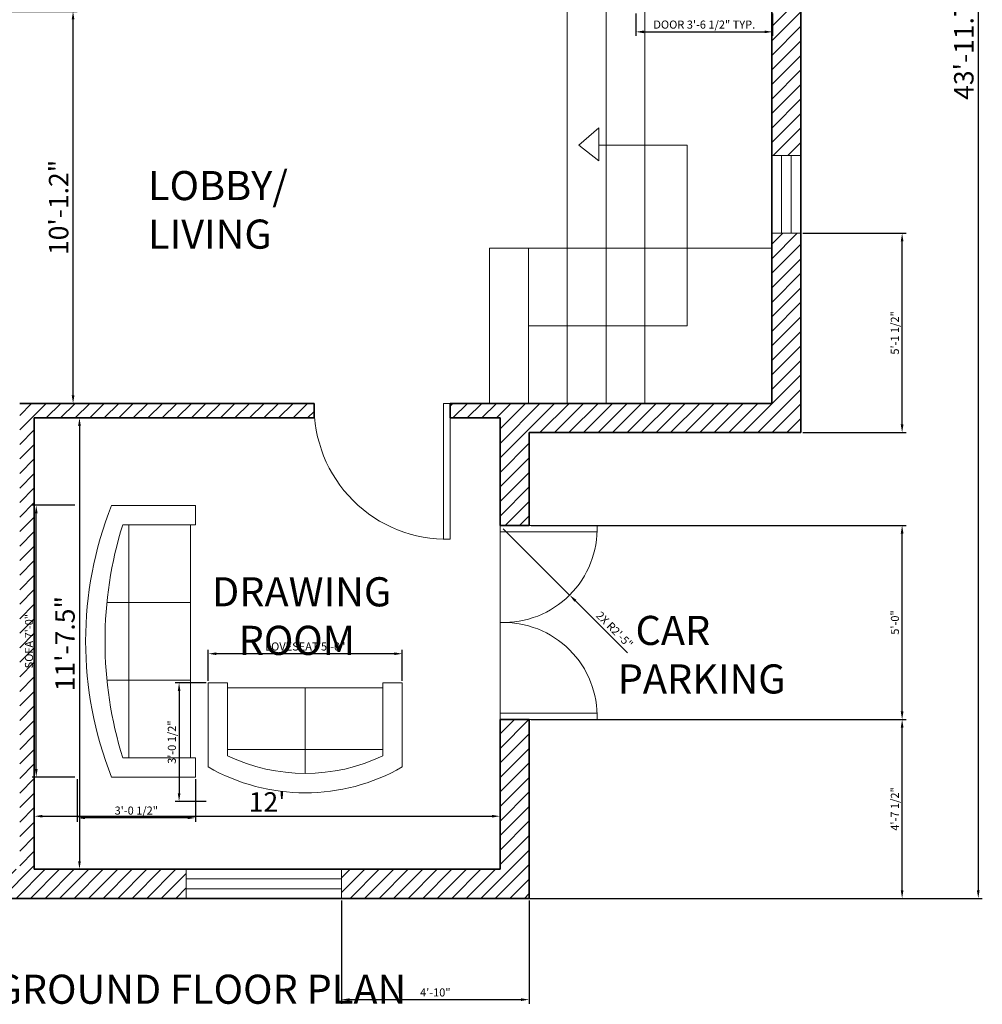
# Model space of a CAD drawing. Units: inches. Extents: x 4740 to 5323, y 7115 to 7713.
# Tile 2 of 6: x 5025 to 5323, y 7115 to 7420. Entities that reach past the tile are written whole.
import ezdxf

# ---------------------------------------------------------------- set-up
doc = ezdxf.new("R2010")
doc.units = ezdxf.units.IN
for name, color, linetype, lineweight in [('A-ANNO-DIMS', 2, 'Continuous', 18), ('A-ANNO-TEXT', 7, 'Continuous', 25), ('A-AREA-IDEN', 7, 'Continuous', 25), ('A-DOOR', 4, 'Continuous', 18), ('A-FLOR-STRS', 7, 'Continuous', 18), ('A-FURN', 8, 'Continuous', 18), ('A-GLAZ', 242, 'Continuous', 18), ('A-WALL', 7, 'Continuous', 35)]:
    doc.layers.add(name, color=color, linetype=linetype, lineweight=lineweight)
doc.layers.add('A-WALL-PATT', color=152, linetype='Continuous', lineweight=13, true_color=0x2776bb)
doc.styles.get("Standard").update_dxf_attribs({"font": 'arial.ttf'})
doc.dimstyles.new('ISO-25', dxfattribs={"dimtxt": 2.5, "dimasz": 2.5, "dimexe": 1.25, "dimexo": 0.625, "dimtad": 1, "dimlunit": 3, "dimtxsty": 'Standard', "dimcen": 2.5, "dimadec": 0, "dimazin": 0, "dimtfac": 1, "dimtmove": 0, "dimatfit": 3, "dimfxl": 1, "dimarcsym": 0})

# ---------------------------------------------------------------- blocks, each defined once
blk = doc.blocks.new('*D23')
at = {"layer": 'A-ANNO-DIMS', "color": 0, "lineweight": -2, "transparency": 16777216}
for p, q in [((5030.58, 7296.66), (5045.19, 7296.66)), ((5043.94, 7294.16), (5043.94, 7159.66)), ((5030.58, 7157.16), (5045.19, 7157.16))]:
    blk.add_line(p, q, dxfattribs=at)
at = {"layer": 'A-ANNO-DIMS', "color": 0, "transparency": 16777216}
for points in [[(5043.52, 7294.16), (5044.36, 7294.16), (5043.94, 7296.66)], [(5043.52, 7159.66), (5044.36, 7159.66), (5043.94, 7157.16)]]:
    blk.add_solid(points, dxfattribs=at)
at = {"layer": 'Defpoints', "color": 0, "transparency": 16777216}
for p in [(5029.96, 7296.66), (5029.96, 7157.16), (5043.94, 7157.16)]:
    blk.add_point(p, dxfattribs=at)
at = {"layer": 'A-ANNO-DIMS', "color": 0, "transparency": 16777216, "insert": (5040.25, 7226.91), "char_height": 6, "attachment_point": 5, "rotation": 90}
blk.add_mtext('11\'-7.5"', dxfattribs=at)
blk = doc.blocks.new('*D24')
at = {"layer": 'A-ANNO-DIMS', "color": 0, "lineweight": -2, "transparency": 16777216}
for p, q in [((5029.96, 7157.78), (5029.96, 7174.81)), ((5173.96, 7157.78), (5173.96, 7174.81)), ((5032.46, 7173.56), (5171.46, 7173.56))]:
    blk.add_line(p, q, dxfattribs=at)
at = {"layer": 'A-ANNO-DIMS', "color": 0, "transparency": 16777216}
for points in [[(5032.46, 7173.97), (5032.46, 7173.14), (5029.96, 7173.56)], [(5171.46, 7173.97), (5171.46, 7173.14), (5173.96, 7173.56)]]:
    blk.add_solid(points, dxfattribs=at)
at = {"layer": 'Defpoints', "color": 0, "transparency": 16777216}
for p in [(5173.96, 7173.56), (5029.96, 7157.16), (5173.96, 7157.16)]:
    blk.add_point(p, dxfattribs=at)
at = {"layer": 'A-ANNO-DIMS', "color": 0, "transparency": 16777216, "insert": (5101.96, 7177.19), "char_height": 6, "attachment_point": 5}
blk.add_mtext("12'", dxfattribs=at)
blk = doc.blocks.new('*D29')
at = {"layer": 'A-ANNO-DIMS', "color": 0, "lineweight": -2, "transparency": 16777216}
for p, q in [((5012.58, 7422.36), (5043.21, 7422.36)), ((5041.96, 7303.66), (5041.96, 7419.86)), ((5026.08, 7301.16), (5043.21, 7301.16))]:
    blk.add_line(p, q, dxfattribs=at)
at = {"layer": 'A-ANNO-DIMS', "color": 0, "transparency": 16777216}
for points in [[(5041.54, 7419.86), (5042.38, 7419.86), (5041.96, 7422.36)], [(5041.54, 7303.66), (5042.38, 7303.66), (5041.96, 7301.16)]]:
    blk.add_solid(points, dxfattribs=at)
at = {"layer": 'Defpoints', "color": 0, "transparency": 16777216}
for p in [(5011.96, 7422.36), (5041.96, 7422.36), (5025.46, 7301.16)]:
    blk.add_point(p, dxfattribs=at)
at = {"layer": 'A-ANNO-DIMS', "color": 0, "transparency": 16777216, "insert": (5038.27, 7361.76), "char_height": 6, "attachment_point": 5, "rotation": 90}
blk.add_mtext('10\'-1.2"', dxfattribs=at)
blk = doc.blocks.new('Sofa - Roundback 7 ft.')
for p, q in [((-12.00002, -32.4421), (-12.00003, -6.5971)), ((11.99997, -32.4421), (11.99998, -6.5971)), ((-36.000027, -34), (-36.000027, -11.4696)), ((35.99998, -34), (35.99998, -11.4696)), ((-35.999844, -13.3819), (35.9998, -13.3819)), ((-36.000027, -32.4421), (35.99998, -32.4421))]:
    blk.add_line(p, q)
for points in [[(-36.000027, -34), (-42.000027, -34), (-42.000027, -8)], [(41.99998, -8), (41.99998, -34), (35.99998, -34)]]:
    blk.add_lwpolyline(points)
for centre, radius, start, end in [((0, -114.25), 114.25, 68.43141, 111.5686), ((-0.00001, -127.1968), 121.1968, 72.72033, 107.2797)]:
    blk.add_arc(centre, radius, start, end)
blk = doc.blocks.new('Sofa - Roundback Loveseat 5 ft.')
for p, q in [((0, -32.44198), (0, -5.99998)), ((-24, -33.99998), (-24, -11.46958)), ((24.00004, -33.99998), (24.00004, -11.46958)), ((-23.9998, -13.38178), (23.99986, -13.38178)), ((-24, -32.44198), (24.00004, -32.44198))]:
    blk.add_line(p, q)
for points in [[(-24, -33.99998), (-30, -33.99998), (-30, -7.99998)], [(30.00004, -7.99998), (30.00004, -33.99998), (24.00004, -33.99998)]]:
    blk.add_lwpolyline(points)
for centre, radius, start, end in [((0, -60.24998), 60.24998, 60.13715, 119.8628), ((0, -61.38438), 55.38444, 64.32083, 115.6792)]:
    blk.add_arc(centre, radius, start, end)
blk = doc.blocks.new('*D36')
at = {"layer": 'A-ANNO-DIMS', "color": 0, "lineweight": -2, "transparency": 16777216}
for p, q in [((5078.58, 7675.86), (5323.05, 7675.86)), ((5321.8, 7673.36), (5321.8, 7150.66)), ((5077.56, 7148.16), (5323.05, 7148.16))]:
    blk.add_line(p, q, dxfattribs=at)
at = {"layer": 'A-ANNO-DIMS', "color": 0, "transparency": 16777216}
for points in [[(5321.38, 7673.36), (5322.22, 7673.36), (5321.8, 7675.86)], [(5321.38, 7150.66), (5322.22, 7150.66), (5321.8, 7148.16)]]:
    blk.add_solid(points, dxfattribs=at)
at = {"layer": 'Defpoints', "color": 0, "transparency": 16777216}
for p in [(5077.96, 7675.86), (5076.93, 7148.16), (5321.8, 7148.16)]:
    blk.add_point(p, dxfattribs=at)
at = {"layer": 'A-ANNO-DIMS', "color": 0, "transparency": 16777216, "insert": (5318.11, 7412.01), "char_height": 6, "attachment_point": 5, "rotation": 90}
blk.add_mtext('43\'-11.7"', dxfattribs=at)
blk = doc.blocks.new('WIN-48IN')
for p, q in [((0, 0), (0, 9)), ((0, 9), (48, 9)), ((48, 9), (48, 0)), ((0, 6), (48, 6)), ((0, 3), (48, 3)), ((48, 0), (0, 0))]:
    blk.add_line(p, q)
blk = doc.blocks.new('WIN-24IN')
for p, q in [((0, 24), (9, 24)), ((0, 24), (0, 0)), ((3, 0), (3, 24)), ((6, 0), (6, 24)), ((9, 0), (9, 24)), ((0, 0), (9, 0))]:
    blk.add_line(p, q)
blk = doc.blocks.new('DOOR-SWING-42IN')
for p, q in [((0, 0), (0, 42)), ((0, 42), (2, 42)), ((2, 42), (2, 0)), ((2, 0), (0, 0))]:
    blk.add_line(p, q)
blk.add_arc((1, 1), 41.01, 358.6028, 91.3972)
blk = doc.blocks.new('*D58')
at = {"layer": 'A-ANNO-DIMS', "color": 0, "lineweight": -2, "transparency": 16777216}
for p, q in [((5215.96, 7421.73), (5215.96, 7414.77)), ((5258.23, 7421.73), (5258.23, 7414.77)), ((5218.46, 7416.02), (5255.73, 7416.02))]:
    blk.add_line(p, q, dxfattribs=at)
at = {"layer": 'A-ANNO-DIMS', "color": 0, "transparency": 16777216}
for points in [[(5218.46, 7416.43), (5218.46, 7415.6), (5215.96, 7416.02)], [(5255.73, 7416.43), (5255.73, 7415.6), (5258.23, 7416.02)]]:
    blk.add_solid(points, dxfattribs=at)
at = {"layer": 'Defpoints', "color": 0, "transparency": 16777216}
for p in [(5215.96, 7422.36), (5258.23, 7422.36), (5258.23, 7416.02)]:
    blk.add_point(p, dxfattribs=at)
at = {"layer": 'A-ANNO-DIMS', "color": 0, "transparency": 16777216, "insert": (5237.1, 7417.94), "char_height": 2.5, "attachment_point": 5}
blk.add_mtext('DOOR 3\'-6 1/2" TYP.', dxfattribs=at)
blk = doc.blocks.new('*D66')
at = {"layer": 'A-ANNO-DIMS', "color": 0, "lineweight": -2, "transparency": 16777216}
for p, q in [((5042.55, 7269.66), (5029.33, 7269.66)), ((5030.58, 7188.16), (5030.58, 7267.16)), ((5042.55, 7185.66), (5029.33, 7185.66))]:
    blk.add_line(p, q, dxfattribs=at)
at = {"layer": 'A-ANNO-DIMS', "color": 0, "transparency": 16777216}
for points in [[(5030.16, 7267.16), (5031, 7267.16), (5030.58, 7269.66)], [(5030.16, 7188.16), (5031, 7188.16), (5030.58, 7185.66)]]:
    blk.add_solid(points, dxfattribs=at)
at = {"layer": 'Defpoints', "color": 0, "transparency": 16777216}
for p in [(5030.58, 7269.66), (5043.18, 7269.66), (5043.18, 7185.66)]:
    blk.add_point(p, dxfattribs=at)
at = {"layer": 'A-ANNO-DIMS', "color": 0, "transparency": 16777216, "insert": (5028.66, 7227.66), "char_height": 2.5, "attachment_point": 5, "rotation": 90}
blk.add_mtext('SOFA 7\'-0"', dxfattribs=at)
blk = doc.blocks.new('*D67')
at = {"layer": 'A-ANNO-DIMS', "color": 0, "lineweight": -2, "transparency": 16777216}
for p, q in [((5043.18, 7185.03), (5043.18, 7171.81)), ((5079.85, 7185.03), (5079.85, 7171.81)), ((5077.35, 7173.06), (5045.68, 7173.06))]:
    blk.add_line(p, q, dxfattribs=at)
at = {"layer": 'A-ANNO-DIMS', "color": 0, "transparency": 16777216}
for points in [[(5045.68, 7173.47), (5045.68, 7172.64), (5043.18, 7173.06)], [(5077.35, 7173.47), (5077.35, 7172.64), (5079.85, 7173.06)]]:
    blk.add_solid(points, dxfattribs=at)
at = {"layer": 'Defpoints', "color": 0, "transparency": 16777216}
for p in [(5043.18, 7185.66), (5079.85, 7185.66), (5043.18, 7173.06)]:
    blk.add_point(p, dxfattribs=at)
at = {"layer": 'A-ANNO-DIMS', "color": 0, "transparency": 16777216, "insert": (5061.51, 7174.97), "char_height": 2.5, "attachment_point": 5}
blk.add_mtext('3\'-0 1/2"', dxfattribs=at)
blk = doc.blocks.new('*D68')
at = {"layer": 'A-ANNO-DIMS', "color": 0, "lineweight": -2, "transparency": 16777216}
for p, q in [((5083.74, 7215.41), (5083.74, 7225.04)), ((5141.24, 7223.79), (5086.24, 7223.79)), ((5143.74, 7215.41), (5143.74, 7225.04))]:
    blk.add_line(p, q, dxfattribs=at)
at = {"layer": 'A-ANNO-DIMS', "color": 0, "transparency": 16777216}
for points in [[(5086.24, 7224.2), (5086.24, 7223.37), (5083.74, 7223.79)], [(5141.24, 7224.2), (5141.24, 7223.37), (5143.74, 7223.79)]]:
    blk.add_solid(points, dxfattribs=at)
at = {"layer": 'Defpoints', "color": 0, "transparency": 16777216}
for p in [(5083.74, 7223.79), (5083.74, 7214.79), (5143.74, 7214.79)]:
    blk.add_point(p, dxfattribs=at)
at = {"layer": 'A-ANNO-DIMS', "color": 0, "transparency": 16777216, "insert": (5113.74, 7225.7), "char_height": 2.5, "attachment_point": 5}
blk.add_mtext('LOVESEAT 5\'-0"', dxfattribs=at)
blk = doc.blocks.new('*D69')
at = {"layer": 'A-ANNO-DIMS', "color": 0, "lineweight": -2, "transparency": 16777216}
for p, q in [((5083.12, 7214.79), (5073.49, 7214.79)), ((5074.74, 7212.29), (5074.74, 7180.62)), ((5083.12, 7178.12), (5073.49, 7178.12))]:
    blk.add_line(p, q, dxfattribs=at)
at = {"layer": 'A-ANNO-DIMS', "color": 0, "transparency": 16777216}
for points in [[(5074.33, 7212.29), (5075.16, 7212.29), (5074.74, 7214.79)], [(5074.33, 7180.62), (5075.16, 7180.62), (5074.74, 7178.12)]]:
    blk.add_solid(points, dxfattribs=at)
at = {"layer": 'Defpoints', "color": 0, "transparency": 16777216}
for p in [(5083.74, 7214.79), (5074.74, 7178.12), (5083.74, 7178.12)]:
    blk.add_point(p, dxfattribs=at)
at = {"layer": 'A-ANNO-DIMS', "color": 0, "transparency": 16777216, "insert": (5072.83, 7196.45), "char_height": 2.5, "attachment_point": 5, "rotation": 90}
blk.add_mtext('3\'-0 1/2"', dxfattribs=at)
blk = doc.blocks.new('*D72')
at = {"layer": 'A-ANNO-DIMS', "color": 0, "lineweight": -2, "transparency": 16777216}
for p, q in [((5124.93, 7147.53), (5124.93, 7115.61)), ((5182.96, 7147.53), (5182.96, 7115.61)), ((5127.43, 7116.86), (5180.46, 7116.86))]:
    blk.add_line(p, q, dxfattribs=at)
at = {"layer": 'A-ANNO-DIMS', "color": 0, "transparency": 16777216}
for points in [[(5127.43, 7117.27), (5127.43, 7116.44), (5124.93, 7116.86)], [(5180.46, 7117.27), (5180.46, 7116.44), (5182.96, 7116.86)]]:
    blk.add_solid(points, dxfattribs=at)
at = {"layer": 'Defpoints', "color": 0, "transparency": 16777216}
for p in [(5124.93, 7148.16), (5182.96, 7148.16), (5182.96, 7116.86)]:
    blk.add_point(p, dxfattribs=at)
at = {"layer": 'A-ANNO-DIMS', "color": 0, "transparency": 16777216, "insert": (5153.95, 7118.76), "char_height": 2.5, "attachment_point": 5}
blk.add_mtext('4\'-10"', dxfattribs=at)
blk = doc.blocks.new('*D76')
at = {"layer": 'A-ANNO-DIMS', "color": 0, "lineweight": -2, "transparency": 16777216}
for p, q in [((5267.58, 7353.76), (5299.51, 7353.76)), ((5298.26, 7294.66), (5298.26, 7351.26)), ((5267.58, 7292.16), (5299.51, 7292.16))]:
    blk.add_line(p, q, dxfattribs=at)
at = {"layer": 'A-ANNO-DIMS', "color": 0, "transparency": 16777216}
for points in [[(5297.84, 7351.26), (5298.68, 7351.26), (5298.26, 7353.76)], [(5297.84, 7294.66), (5298.68, 7294.66), (5298.26, 7292.16)]]:
    blk.add_solid(points, dxfattribs=at)
at = {"layer": 'Defpoints', "color": 0, "transparency": 16777216}
for p in [(5266.96, 7353.76), (5298.26, 7353.76), (5266.96, 7292.16)]:
    blk.add_point(p, dxfattribs=at)
at = {"layer": 'A-ANNO-DIMS', "color": 0, "transparency": 16777216, "insert": (5296.34, 7322.96), "char_height": 2.5, "attachment_point": 5, "rotation": 90}
blk.add_mtext('5\'-1 1/2"', dxfattribs=at)
blk = doc.blocks.new('*D78')
at = {"layer": 'A-ANNO-DIMS', "color": 0, "lineweight": -2, "transparency": 16777216}
for p, q in [((5183.58, 7203.44), (5299.51, 7203.44)), ((5298.26, 7150.66), (5298.26, 7200.94)), ((5183.58, 7148.16), (5299.51, 7148.16))]:
    blk.add_line(p, q, dxfattribs=at)
at = {"layer": 'A-ANNO-DIMS', "color": 0, "transparency": 16777216}
for points in [[(5297.84, 7200.94), (5298.68, 7200.94), (5298.26, 7203.44)], [(5297.84, 7150.66), (5298.68, 7150.66), (5298.26, 7148.16)]]:
    blk.add_solid(points, dxfattribs=at)
at = {"layer": 'Defpoints', "color": 0, "transparency": 16777216}
for p in [(5182.96, 7203.44), (5298.26, 7203.44), (5182.96, 7148.16)]:
    blk.add_point(p, dxfattribs=at)
at = {"layer": 'A-ANNO-DIMS', "color": 0, "transparency": 16777216, "insert": (5296.34, 7175.8), "char_height": 2.5, "attachment_point": 5, "rotation": 90}
blk.add_mtext('4\'-7 1/2"', dxfattribs=at)
blk = doc.blocks.new('*D79')
at = {"layer": 'A-ANNO-DIMS', "color": 0, "lineweight": -2, "transparency": 16777216}
for p, q in [((5183.58, 7263.44), (5299.51, 7263.44)), ((5298.26, 7205.94), (5298.26, 7260.94)), ((5183.58, 7203.44), (5299.51, 7203.44))]:
    blk.add_line(p, q, dxfattribs=at)
at = {"layer": 'A-ANNO-DIMS', "color": 0, "transparency": 16777216}
for points in [[(5297.84, 7260.94), (5298.68, 7260.94), (5298.26, 7263.44)], [(5297.84, 7205.94), (5298.68, 7205.94), (5298.26, 7203.44)]]:
    blk.add_solid(points, dxfattribs=at)
at = {"layer": 'Defpoints', "color": 0, "transparency": 16777216}
for p in [(5182.96, 7263.44), (5298.26, 7263.44), (5182.96, 7203.44)]:
    blk.add_point(p, dxfattribs=at)
at = {"layer": 'A-ANNO-DIMS', "color": 0, "transparency": 16777216, "insert": (5296.36, 7233.44), "char_height": 2.5, "attachment_point": 5, "rotation": 90}
blk.add_mtext('5\'-0"', dxfattribs=at)
blk = doc.blocks.new('*D92')
at = {"layer": 'A-ANNO-DIMS', "color": 0, "lineweight": -2, "transparency": 16777216}
for p, q in [((5174.96, 7262.44), (5195.48, 7241.92)), ((5213.34, 7224.06), (5197.24, 7240.16))]:
    blk.add_line(p, q, dxfattribs=at)
at = {"layer": 'A-ANNO-DIMS', "color": 0, "transparency": 16777216}
blk.add_solid([(5197.54, 7240.45), (5196.95, 7239.86), (5195.48, 7241.92)], dxfattribs=at)
at = {"layer": 'Defpoints', "color": 0, "transparency": 16777216}
for p in [(5174.96, 7262.44), (5195.48, 7241.92)]:
    blk.add_point(p, dxfattribs=at)
at = {"layer": 'A-ANNO-DIMS', "color": 0, "transparency": 16777216, "insert": (5209.13, 7230.96), "char_height": 2.5, "attachment_point": 5, "rotation": 314.9988}
blk.add_mtext('2X R2\'-5"', dxfattribs=at)

msp = doc.modelspace()

# ---------------------------------------------------------------- hatches: boundary and pattern name
at = {"layer": 'A-WALL-PATT'}
h = msp.add_hatch(dxfattribs=at)
h.set_pattern_fill('ANSI31', color=256)
h.paths.add_polyline_path([(4925.343, 7632.357), (4776.459, 7632.357), (4776.459, 7486.448), (4785.459, 7486.448), (4785.459, 7522.857), (4959.459, 7522.857), (4959.459, 7527.357), (4785.459, 7527.357), (4785.459, 7623.357), (4833.459, 7623.357), (4925.343, 7623.357)])
h.paths.add_polyline_path([(5010.258, 7599.357), (5004.258, 7599.357), (4986.459, 7599.357), (4986.459, 7623.357), (4986.459, 7632.357), (4977.459, 7632.357), (4949.343, 7632.357), (4949.343, 7623.357), (4977.459, 7623.357), (4977.459, 7599.357), (4977.459, 7594.857), (4977.459, 7590.357), (4977.459, 7524.857, -0.0293864), (4977.459, 7522.857), (4977.459, 7426.857), (4977.459, 7422.357), (4977.459, 7419.778), (4981.959, 7419.778), (4981.959, 7422.357), (5041.959, 7422.357), (5041.959, 7479.357), (5037.459, 7479.357), (5037.459, 7426.857), (4981.959, 7426.857), (4981.959, 7590.357), (5010.258, 7590.357)])
h.paths.add_polyline_path([(5086.959, 7666.857), (5206.959, 7666.857), (5206.959, 7646.624), (5215.959, 7646.624), (5215.959, 7675.857), (5077.959, 7675.857), (5077.959, 7599.357), (5046.258, 7599.357), (5046.258, 7590.357), (5082.459, 7590.357), (5082.459, 7474.857, -0.0106371), (5084.459, 7474.857), (5086.959, 7474.857)])
h.paths.add_polyline_path([(5215.959, 7610.624), (5206.959, 7610.624), (5206.959, 7594.857), (5104.959, 7594.857), (5104.959, 7592.357, -0.0293864), (5104.959, 7590.357), (5206.959, 7590.357), (5206.959, 7426.857), (5104.959, 7426.857), (5082.459, 7426.857), (5082.459, 7422.357), (5104.959, 7422.357), (5215.959, 7422.357), (5215.959, 7464.357), (5215.959, 7506.357)])
h.paths.add_polyline_path([(4881.459, 7375.857), (4977.459, 7375.857), (4977.459, 7296.657), (4981.959, 7296.657), (4981.959, 7384.857), (4951.959, 7384.857), (4785.459, 7384.857), (4785.459, 7438.448), (4776.459, 7438.448), (4776.459, 7375.857), (4872.459, 7375.857), (4872.459, 7337.044), (4881.459, 7337.044)])
h.paths.add_polyline_path([(4881.459, 7313.044), (4872.459, 7313.044), (4872.459, 7148.157), (4916.568, 7148.157), (4916.568, 7157.157), (4881.459, 7157.157), (4881.459, 7269.357), (4981.959, 7269.357), (4981.959, 7273.857), (4963.959, 7273.857), (4881.459, 7273.857)])
h.paths.add_polyline_path([(5029.959, 7296.657), (5116.509, 7296.657), (5116.509, 7299.157, -0.0121933), (5116.509, 7301.157), (5025.459, 7301.157), (5025.459, 7157.157), (4964.568, 7157.157), (4964.568, 7148.157), (5076.933, 7148.157), (5076.933, 7157.157), (5029.959, 7157.157)])
h.paths.add_polyline_path([(5182.959, 7203.442), (5173.959, 7203.442), (5173.959, 7157.157), (5124.933, 7157.157), (5124.933, 7148.157), (5182.959, 7148.157)])
h.paths.add_polyline_path([(5266.959, 7353.764), (5257.959, 7353.764), (5257.959, 7301.157), (5182.959, 7301.157), (5158.509, 7301.157), (5158.509, 7296.657), (5173.959, 7296.657), (5173.959, 7263.442), (5182.959, 7263.442), (5182.959, 7292.157), (5266.959, 7292.157)])
h.paths.add_polyline_path([(5266.959, 7422.357), (5257.959, 7422.357), (5257.959, 7377.764), (5266.959, 7377.764)])

# ---------------------------------------------------------------- linework, layer by layer
at = {"layer": 'A-DOOR'}
for p, q in [((5173.959, 7263.442), (5173.959, 7203.442)), ((5173.959, 7263.442), (5203.959, 7263.442)), ((5203.959, 7263.442), (5203.959, 7261.442)), ((5203.959, 7261.442), (5173.959, 7261.442)), ((5173.959, 7203.442), (5173.959, 7233.442)), ((5203.959, 7205.442), (5173.959, 7205.442)), ((5203.959, 7203.442), (5203.959, 7205.442)), ((5173.959, 7203.442), (5203.959, 7203.442))]:
    msp.add_line(p, q, dxfattribs=at)
for centre, start, end in [((5174.959, 7262.442), 268.02507, 1.97493), ((5174.959, 7204.442), 358.02507, 91.97493)]:
    msp.add_arc(centre, 29.017, start, end, dxfattribs=at)
at = {"layer": 'A-FLOR-STRS'}
for p, q in [((5194.734, 7301.157), (5194.734, 7422.357)), ((5206.734, 7301.157), (5206.734, 7422.357)), ((5218.734, 7301.157), (5218.734, 7422.357)), ((5204.502, 7386.398), (5198.277, 7380.977)), ((5204.502, 7380.977), (5204.502, 7386.398)), ((5198.277, 7380.977), (5204.502, 7376.126)), ((5231.831, 7380.977), (5204.502, 7380.977)), ((5204.502, 7376.126), (5204.502, 7380.977)), ((5231.831, 7325.157), (5231.831, 7380.977)), ((5257.959, 7349.157), (5170.734, 7349.157)), ((5170.734, 7301.157), (5170.734, 7349.157)), ((5182.734, 7301.157), (5182.734, 7349.157)), ((5182.959, 7349.157), (5257.959, 7349.157)), ((5182.734, 7325.157), (5231.831, 7325.157))]:
    msp.add_line(p, q, dxfattribs=at)
at = {"layer": 'A-WALL'}
for p, q in [((5257.959, 7422.357), (5257.959, 7301.157)), ((5266.959, 7422.357), (5266.959, 7292.157)), ((5116.509, 7301.157), (5025.459, 7301.157)), ((5116.509, 7301.157), (5116.509, 7296.657)), ((5182.959, 7301.157), (5158.509, 7301.157)), ((5158.509, 7301.157), (5158.509, 7296.657)), ((5182.959, 7301.157), (5257.959, 7301.157)), ((5029.959, 7296.657), (5029.959, 7157.157)), ((5116.509, 7296.657), (5029.959, 7296.657)), ((5173.959, 7296.657), (5158.509, 7296.657)), ((5173.959, 7296.657), (5173.959, 7263.442)), ((5182.959, 7292.157), (5182.959, 7263.442)), ((5182.959, 7292.157), (5266.959, 7292.157)), ((5173.959, 7263.442), (5182.959, 7263.442)), ((5173.959, 7203.442), (5182.959, 7203.442)), ((5173.959, 7203.442), (5173.959, 7157.157)), ((5182.959, 7203.442), (5182.959, 7148.157)), ((5173.959, 7157.157), (5029.959, 7157.157)), ((5182.959, 7148.157), (4872.459, 7148.157))]:
    msp.add_line(p, q, dxfattribs=at)

# ---------------------------------------------------------------- block references
at = {"layer": 'A-DOOR', "rotation": 180}
msp.add_blockref('DOOR-SWING-42IN', (5158.509, 7301.157), dxfattribs=at)
at = {"layer": 'A-FURN'}
for name, p, rotation in [('Sofa - Roundback 7 ft.', (5045.845, 7227.656), 90), ('Sofa - Roundback Loveseat 5 ft.', (5113.744, 7180.786), 180)]:
    msp.add_blockref(name, p, dxfattribs=dict(at, rotation=rotation))
at = {"layer": 'A-GLAZ'}
for name, p in [('WIN-24IN', (5257.959, 7353.764)), ('WIN-48IN', (5076.933, 7148.157))]:
    msp.add_blockref(name, p, dxfattribs=at)

# ---------------------------------------------------------------- texts
at = {"layer": 'A-ANNO-TEXT', "insert": (5014.915, 7124.575), "char_height": 9, "attachment_point": 1}
msp.add_mtext_dynamic_manual_height_columns('{ GROUND FLOOR PLAN}', width=334.1036, gutter_width=12.5, heights=[49.338], dxfattribs=at)
at = {"layer": 'A-AREA-IDEN', "char_height": 9, "attachment_point": 1}
for s, insert in [('{ LOBBY/\\P LIVING}', (5062.38, 7372.996)), ('{DRAWING\\P   ROOM}', (5084.896, 7247.427)), ('{  CAR PARKING}', (5210.34, 7235.493))]:
    msp.add_mtext_dynamic_manual_height_columns(s, width=75.84022, gutter_width=12.5, heights=[0], dxfattribs=dict(at, insert=insert))

# ---------------------------------------------------------------- dimensions: what is measured, and where the dimension line sits
at = {"layer": 'A-ANNO-DIMS'}
for base, p1, p2, angle, override, picture, middle in [((5321.801, 7148.157), (5077.959, 7675.857), (5076.933, 7148.157), 90, {"dimtxt": 6, "dimclrd": 0, "dimclre": 0, "dimclrt": 0}, '*D36', (5318.111, 7412.007)), ((5041.959, 7422.357), (5025.459, 7301.157), (5011.959, 7422.357), 90, {"dimtxt": 6, "dimclrd": 0, "dimclre": 0, "dimclrt": 0}, '*D29', (5038.271, 7361.757)), ((5298.259, 7353.764), (5266.959, 7292.157), (5266.959, 7353.764), 90, {"dimdec": 1, "dimlfac": 1, "dimrnd": 0, "dimzin": 1, "dimdsep": 46, "dimlunit": 4, "dimfrac": 2}, '*D76', (5296.342, 7322.961)), ((5043.939, 7157.157), (5029.959, 7296.657), (5029.959, 7157.157), 90, {"dimtxt": 6, "dimclrd": 0, "dimclre": 0, "dimclrt": 0}, '*D23', (5040.251, 7226.907)), ((5298.259, 7263.442), (5182.959, 7203.442), (5182.959, 7263.442), 90, {"dimdec": 1, "dimlfac": 1, "dimrnd": 0, "dimzin": 1, "dimdsep": 46, "dimlunit": 4, "dimfrac": 2}, '*D79', (5296.358, 7233.442)), ((5074.744, 7178.12), (5083.744, 7214.786), (5083.744, 7178.12), 270, {"dimdec": 1, "dimlfac": 1, "dimrnd": 0, "dimzin": 1, "dimdsep": 46, "dimlunit": 4, "dimfrac": 2}, '*D69', (5072.826, 7196.453)), ((5298.259, 7203.442), (5182.959, 7148.157), (5182.959, 7203.442), 90, {"dimdec": 1, "dimlfac": 1, "dimrnd": 0, "dimzin": 1, "dimdsep": 46, "dimlunit": 4, "dimfrac": 2}, '*D78', (5296.342, 7175.799)), ((5043.179, 7173.056), (5079.845, 7185.656), (5043.179, 7185.656), 180, {"dimdec": 1, "dimlfac": 1, "dimrnd": 0, "dimzin": 1, "dimdsep": 46, "dimlunit": 4, "dimfrac": 2}, '*D67', (5061.512, 7174.974))]:
    dim = msp.add_linear_dim(base=base, p1=p1, p2=p2, angle=angle, dimstyle='ISO-25', override=override, dxfattribs=at)
    dim.commit()
    dim.dimension.update_dxf_attribs({"geometry": picture, "text_midpoint": middle})
dim = msp.add_linear_dim(base=(5258.233, 7416.016), p1=(5215.959, 7422.357), p2=(5258.233, 7422.357), text='DOOR <> TYP.', dimstyle='ISO-25', override={"dimdec": 1, "dimlfac": 1, "dimrnd": 0, "dimzin": 1, "dimdsep": 46, "dimlunit": 4, "dimfrac": 2}, dxfattribs=at)
dim.commit()
dim.dimension.update_dxf_attribs({"geometry": '*D58', "text_midpoint": (5237.096, 7417.935)})
for base, p1, p2, angle, text, picture, middle in [((5030.579, 7269.656), (5043.179, 7185.656), (5043.179, 7269.656), 90, 'SOFA <>', '*D66', (5028.66, 7227.656)), ((5083.744, 7223.786), (5143.744, 7214.786), (5083.744, 7214.786), 180, 'LOVESEAT <>', '*D68', (5113.744, 7225.705))]:
    dim = msp.add_linear_dim(base=base, p1=p1, p2=p2, angle=angle, text=text, dimstyle='ISO-25', override={"dimdec": 1, "dimlfac": 1, "dimrnd": 0, "dimzin": 1, "dimdsep": 46, "dimlunit": 4, "dimfrac": 2}, dxfattribs=at)
    dim.commit()
    dim.dimension.update_dxf_attribs({"geometry": picture, "text_midpoint": middle})
dim = msp.add_radius_dim(center=(5174.959, 7262.442), mpoint=(5195.477, 7241.923), text='2X <>', dimstyle='ISO-25', override={"dimdec": 1, "dimlfac": 1, "dimrnd": 0, "dimzin": 1, "dimdsep": 46, "dimlunit": 4, "dimfrac": 2}, dxfattribs=at)
dim.commit()
dim.dimension.update_dxf_attribs({"geometry": '*D92', "text_midpoint": (5207.788, 7229.612), "dimtype": 164})
for base, p1, p2, override, picture, middle in [((5173.959, 7173.556), (5029.959, 7157.157), (5173.959, 7157.157), {"dimtxt": 6, "dimclrd": 0, "dimclre": 0, "dimclrt": 0}, '*D24', (5101.959, 7177.194)), ((5182.959, 7116.857), (5124.933, 7148.157), (5182.959, 7148.157), {"dimdec": 1, "dimlfac": 1, "dimrnd": 0, "dimzin": 1, "dimdsep": 46, "dimlunit": 4, "dimfrac": 2}, '*D72', (5153.946, 7118.758))]:
    dim = msp.add_linear_dim(base=base, p1=p1, p2=p2, dimstyle='ISO-25', override=override, dxfattribs=at)
    dim.commit()
    dim.dimension.update_dxf_attribs({"geometry": picture, "text_midpoint": middle})

doc.saveas('drawing.dxf')
